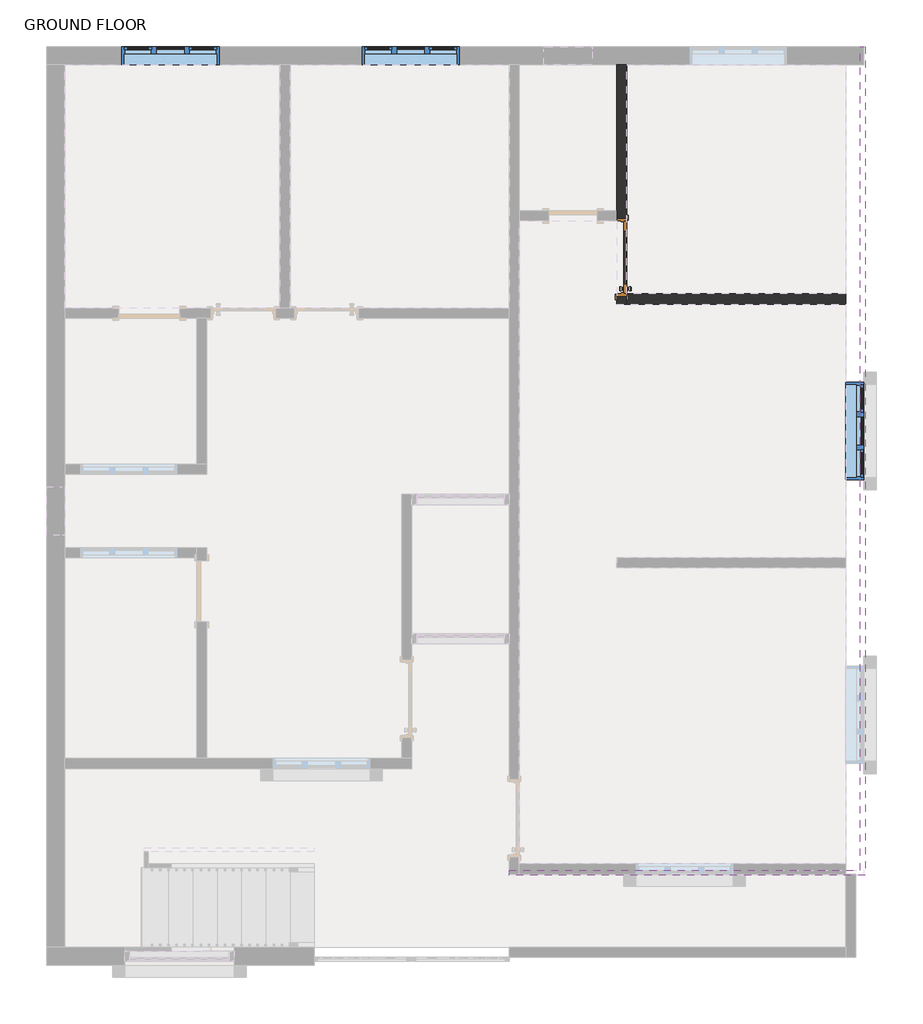
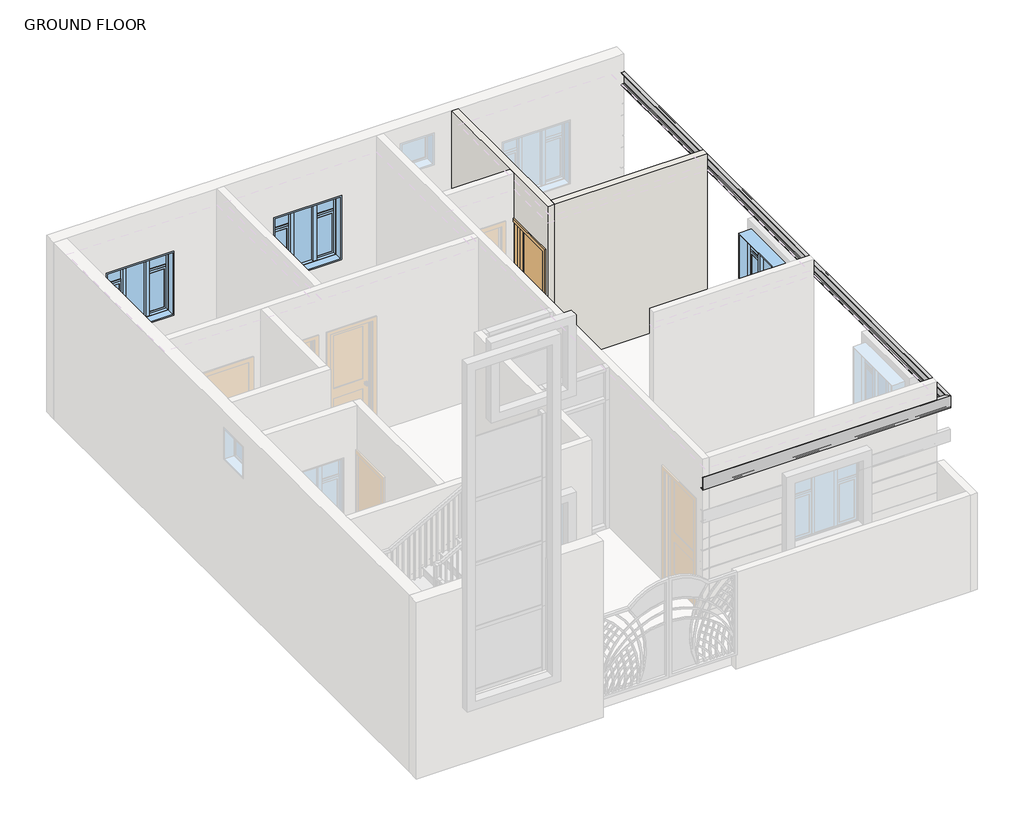
# One storey, part 4 of 7: 3 windows, 2 walls, 1 door, 1 proxy.
"""IFC4 building model written with IfcOpenShell, lengths in millimetres."""

from ifc_helpers import new_model, si_unit, frame, origin, place, context, project, spatial, polyline, circle_curve, ellipse_curve, faceted_brep, transform, mapped, element, save
from ifc_brep_helpers import plane_surface, cylinder_surface, revolved_surface, advanced_brep
from components import door_2e56f206, window_casement_triple_side_transom_window_4_x_4_fd24aed3

model = new_model("IFC4")

# Units and contexts
model_context = context("Model", 3, world=origin())
ifc_project = project(units=[si_unit("LENGTHUNIT", "METRE", prefix="MILLI")], contexts=[model_context])

# Site, building, storey
site = spatial("IfcSite", under=ifc_project)
building = spatial("IfcBuilding", under=site)
storey = spatial("IfcBuildingStorey", under=building, Name="GROUND FLOOR", Elevation=304.8)

# Proxy
placement = place(None, origin())
element("IfcBuildingElementProxy", 1, Name="Reveal", ObjectType="Reveal", at=placement, inside=storey, context=model_context, shape_type="AdvancedBrep", body=[
    advanced_brep(
    [(-9198.1023867, -1857.2343863, 3009.9), (-9198.1023867, -1793.9883863, 3009.9), (-9198.1023867, -1793.9883863, 3008.5203242), (-9198.1023867, -1798.3711955, 3003.3465897), (-9198.1023867, -1821.9918863, 2999.4098), (-9198.1023867, -1841.2297679, 2996.20348), (-9198.1023867, -1849.9953863, 2985.856011), (-9198.1023867, -1849.9953863, 2805.343989), (-9198.1023867, -1841.2297679, 2794.99652), (-9198.1023867, -1821.9918863, 2791.7902), (-9198.1023867, -1798.3711955, 2787.8534103), (-9198.1023867, -1793.9883863, 2782.6796758), (-9198.1023867, -1793.9883863, 2781.3), (-9198.1023867, -1857.2343863, 2781.3), (-4738.2179867, -1857.2343863, 3009.9), (-4738.2179867, -1857.2343863, 2781.3), (-4801.4639867, -1793.9883863, 2781.3), (-4801.4639867, -1793.9883863, 2782.6796758), (-4797.0811775, -1798.3711955, 2787.8534103), (-4773.4604867, -1821.9918863, 2791.7902), (-4754.2226051, -1841.2297679, 2794.99652), (-4745.4569867, -1849.9953863, 2805.343989), (-4745.4569867, -1849.9953863, 2985.856011), (-4754.2226051, -1841.2297679, 2996.20348), (-4773.4604867, -1821.9918863, 2999.4098), (-4797.0811775, -1798.3711955, 3003.3465897), (-4801.4639867, -1793.9883863, 3008.5203242), (-4801.4639867, -1793.9883863, 3009.9)],
    [
        (0, 1),
        (1, 2),
        (2, 3, circle_curve(frame((-9198.1023867, -1799.2334863, 3008.5203242), z_axis=(-1.0, 0.0, 0.0), x_axis=(0.0, 1.0, 0.0)), 5.2451)),
        (3, 4),
        (4, 5),
        (5, 6, circle_curve(frame((-9198.1023867, -1839.5051863, 2985.856011), z_axis=(1.0, 0.0, 0.0), x_axis=(0.0, 1.0, 0.0)), 10.4902)),
        (6, 7),
        (7, 8, circle_curve(frame((-9198.1023867, -1839.5051863, 2805.343989), z_axis=(1.0, 0.0, 0.0), x_axis=(0.0, 1.0, 0.0)), 10.4902)),
        (8, 9),
        (9, 10),
        (10, 11, circle_curve(frame((-9198.1023867, -1799.2334863, 2782.6796758), z_axis=(-1.0, 0.0, 0.0), x_axis=(0.0, 1.0, 0.0)), 5.2451)),
        (11, 12),
        (12, 13),
        (13, 0),
        (14, 15),
        (15, 16),
        (16, 17),
        (17, 18, ellipse_curve(frame((-4796.2188867, -1799.2334863, 2782.6796758), z_axis=(0.7071067811865498, 0.7071067811865454, 0.0), x_axis=(-0.7071067811865451, 0.7071067811865498, 0.0)), 7.4176916, 5.2451)),
        (18, 19),
        (19, 20),
        (20, 21, ellipse_curve(frame((-4755.9471867, -1839.5051863, 2805.343989), z_axis=(-0.7071067811865498, -0.7071067811865454, 0.0), x_axis=(0.7071067811865451, -0.7071067811865498, 0.0)), 14.8353831, 10.4902)),
        (21, 22),
        (22, 23, ellipse_curve(frame((-4755.9471867, -1839.5051863, 2985.856011), z_axis=(-0.7071067811865498, -0.7071067811865454, 0.0), x_axis=(0.7071067811865451, -0.7071067811865498, 0.0)), 14.8353831, 10.4902)),
        (23, 24),
        (24, 25),
        (25, 26, ellipse_curve(frame((-4796.2188867, -1799.2334863, 3008.5203242), z_axis=(0.7071067811865498, 0.7071067811865454, 0.0), x_axis=(-0.7071067811865451, 0.7071067811865498, 0.0)), 7.4176916, 5.2451)),
        (26, 27),
        (27, 14),
        (0, 14),
        (27, 1),
        (26, 2),
        (25, 3),
        (24, 4),
        (23, 5),
        (22, 6),
        (21, 7),
        (20, 8),
        (19, 9),
        (18, 10),
        (17, 11),
        (16, 12),
        (15, 13),
    ],
    [
        plane_surface(frame((-9198.1023867, 8292.2500137, 304.8), z_axis=(-1.0, 0.0, 0.0), x_axis=(0.0, -1.0, 0.0))),
        plane_surface(frame((-4753.1023867, -1842.3499863, 2590.8), z_axis=(0.7071067811865498, 0.7071067811865454, 0.0), x_axis=(-0.7071067811865454, 0.7071067811865498, 0.0))),
        plane_surface(frame((-9198.1023867, -1857.2343863, 3009.9), z_axis=(0.0, 0.0, 1.0), x_axis=(1.0, 0.0, 0.0))),
        plane_surface(frame((-9198.1023867, -1793.9883863, 3009.9), z_axis=(0.0, 1.0, 0.0), x_axis=(1.0, 0.0, 0.0))),
        cylinder_surface(frame((-9198.1023867, -1799.2334863, 3008.5203242), z_axis=(-1.0, 0.0, 0.0), x_axis=(0.0, 1.0, 0.0)), 5.2451),
        plane_surface(frame((-9198.1023867, -1798.3711955, 3003.3465897), z_axis=(0.0, 0.16439930721687082, -0.9863938705135049), x_axis=(1.0, 0.0, 0.0))),
        plane_surface(frame((-9198.1023867, -1821.9918863, 2999.4098), z_axis=(0.0, 0.16439930721687146, -0.9863938705135048), x_axis=(1.0, 0.0, 0.0))),
        revolved_surface(polyline([(-4745.4569867, -1829.0149863000001, 2985.856011), (-9198.1023867, -1829.0149863000001, 2985.856011)]), (-9198.1023867, -1839.5051863, 2985.856011), (1.0, 0.0, 0.0)),
        plane_surface(frame((-9198.1023867, -1849.9953863, 2985.856011), z_axis=(0.0, 1.0, 0.0), x_axis=(1.0, 0.0, 0.0))),
        revolved_surface(polyline([(-4745.4569867, -1829.0149863000001, 2805.343989), (-9198.1023867, -1829.0149863000001, 2805.343989)]), (-9198.1023867, -1839.5051863, 2805.343989), (1.0, 0.0, 0.0)),
        plane_surface(frame((-9198.1023867, -1841.2297679, 2794.99652), z_axis=(0.0, 0.1643993072168769, 0.9863938705135039), x_axis=(1.0, 0.0, 0.0))),
        plane_surface(frame((-9198.1023867, -1821.9918863, 2791.7902), z_axis=(0.0, 0.16439930721687793, 0.9863938705135037), x_axis=(1.0, 0.0, 0.0))),
        cylinder_surface(frame((-9198.1023867, -1799.2334863, 2782.6796758), z_axis=(-1.0, 0.0, 0.0), x_axis=(0.0, 1.0, 0.0)), 5.2451),
        plane_surface(frame((-9198.1023867, -1793.9883863, 2782.6796758), z_axis=(0.0, 1.0, 0.0), x_axis=(1.0, 0.0, 0.0))),
        plane_surface(frame((-9198.1023867, -1793.9883863, 2781.3), z_axis=(0.0, 0.0, -1.0), x_axis=(1.0, 0.0, 0.0))),
        plane_surface(frame((-9198.1023867, -1857.2343863, 2781.3), z_axis=(0.0, -1.0, 0.0), x_axis=(1.0, 0.0, 0.0))),
    ],
    [
        (0, [[1, 2, 3, 4, 5, 6, 7, 8, 9, 10, 11, 12, 13, 14]]),
        (1, [[15, 16, 17, 18, 19, 20, 21, 22, 23, 24, 25, 26, 27, 28]]),
        (2, [[-1, 29, -28, 30]]),
        (3, [[-2, -30, -27, 31]]),
        (4, [[-3, -31, -26, 32]]),
        (5, [[-4, -32, -25, 33]]),
        (6, [[-5, -33, -24, 34]]),
        (7, [[-6, -34, -23, 35]]),
        (8, [[-7, -35, -22, 36]]),
        (9, [[-8, -36, -21, 37]]),
        (10, [[-9, -37, -20, 38]]),
        (11, [[-10, -38, -19, 39]]),
        (12, [[-11, -39, -18, 40]]),
        (13, [[-12, -40, -17, 41]]),
        (14, [[-13, -41, -16, 42]]),
        (15, [[-14, -42, -15, -29]]),
    ],
),
    advanced_brep(
    [(-4738.2179867, 8520.8500137, 3009.9), (-4738.2179867, 8520.8500137, 2781.3), (-4801.4639867, 8520.8500137, 2781.3), (-4801.4639867, 8520.8500137, 2782.6796758), (-4797.0811775, 8520.8500137, 2787.8534103), (-4773.4604867, 8520.8500137, 2791.7902), (-4754.2226051, 8520.8500137, 2794.99652), (-4745.4569867, 8520.8500137, 2805.343989), (-4745.4569867, 8520.8500137, 2985.856011), (-4754.2226051, 8520.8500137, 2996.20348), (-4773.4604867, 8520.8500137, 2999.4098), (-4797.0811775, 8520.8500137, 3003.3465897), (-4801.4639867, 8520.8500137, 3008.5203242), (-4801.4639867, 8520.8500137, 3009.9), (-4738.2179867, -1857.2343863, 3009.9), (-4801.4639867, -1793.9883863, 3009.9), (-4801.4639867, -1793.9883863, 3008.5203242), (-4797.0811775, -1798.3711955, 3003.3465897), (-4773.4604867, -1821.9918863, 2999.4098), (-4754.2226051, -1841.2297679, 2996.20348), (-4745.4569867, -1849.9953863, 2985.856011), (-4745.4569867, -1849.9953863, 2805.343989), (-4754.2226051, -1841.2297679, 2794.99652), (-4773.4604867, -1821.9918863, 2791.7902), (-4797.0811775, -1798.3711955, 2787.8534103), (-4801.4639867, -1793.9883863, 2782.6796758), (-4801.4639867, -1793.9883863, 2781.3), (-4738.2179867, -1857.2343863, 2781.3)],
    [
        (0, 1),
        (1, 2),
        (2, 3),
        (3, 4, circle_curve(frame((-4796.2188867, 8520.8500137, 2782.6796758), z_axis=(0.0, 1.0, 0.0), x_axis=(-1.0, 0.0, 0.0)), 5.2451)),
        (4, 5),
        (5, 6),
        (6, 7, circle_curve(frame((-4755.9471867, 8520.8500137, 2805.343989), z_axis=(0.0, -1.0, 0.0), x_axis=(-1.0, 0.0, 0.0)), 10.4902)),
        (7, 8),
        (8, 9, circle_curve(frame((-4755.9471867, 8520.8500137, 2985.856011), z_axis=(0.0, -1.0, 0.0), x_axis=(-1.0, 0.0, 0.0)), 10.4902)),
        (9, 10),
        (10, 11),
        (11, 12, circle_curve(frame((-4796.2188867, 8520.8500137, 3008.5203242), z_axis=(0.0, 1.0, 0.0), x_axis=(-1.0, 0.0, 0.0)), 5.2451)),
        (12, 13),
        (13, 0),
        (14, 15),
        (15, 16),
        (16, 17, ellipse_curve(frame((-4796.2188867, -1799.2334863, 3008.5203242), z_axis=(-0.7071067811865498, -0.7071067811865454, 0.0), x_axis=(-0.7071067811865455, 0.7071067811865496, 0.0)), 7.4176916, 5.2451)),
        (17, 18),
        (18, 19),
        (19, 20, ellipse_curve(frame((-4755.9471867, -1839.5051863, 2985.856011), z_axis=(0.7071067811865498, 0.7071067811865454, 0.0), x_axis=(0.7071067811865455, -0.7071067811865496, 0.0)), 14.8353831, 10.4902)),
        (20, 21),
        (21, 22, ellipse_curve(frame((-4755.9471867, -1839.5051863, 2805.343989), z_axis=(0.7071067811865498, 0.7071067811865454, 0.0), x_axis=(0.7071067811865455, -0.7071067811865496, 0.0)), 14.8353831, 10.4902)),
        (22, 23),
        (23, 24),
        (24, 25, ellipse_curve(frame((-4796.2188867, -1799.2334863, 2782.6796758), z_axis=(-0.7071067811865498, -0.7071067811865454, 0.0), x_axis=(-0.7071067811865455, 0.7071067811865496, 0.0)), 7.4176916, 5.2451)),
        (25, 26),
        (26, 27),
        (27, 14),
        (0, 14),
        (27, 1),
        (26, 2),
        (25, 3),
        (24, 4),
        (23, 5),
        (22, 6),
        (21, 7),
        (20, 8),
        (19, 9),
        (18, 10),
        (17, 11),
        (16, 12),
        (15, 13),
    ],
    [
        plane_surface(frame((-14983.6015581, 8520.8500137, 0.0), z_axis=(0.0, 1.0, 0.0), x_axis=(-1.0, 0.0, 0.0))),
        plane_surface(frame((-4753.1023867, -1842.3499863, 3200.4), z_axis=(-0.7071067811865498, -0.7071067811865454, 0.0), x_axis=(-0.7071067811865454, 0.7071067811865498, 0.0))),
        plane_surface(frame((-4738.2179867, 8520.8500137, 3009.9), z_axis=(1.0, 0.0, 0.0), x_axis=(0.0, -1.0, 0.0))),
        plane_surface(frame((-4738.2179867, 8520.8500137, 2781.3), z_axis=(0.0, 0.0, -1.0), x_axis=(0.0, -1.0, 0.0))),
        plane_surface(frame((-4801.4639867, 8520.8500137, 2781.3), z_axis=(-1.0, 0.0, 0.0), x_axis=(0.0, -1.0, 0.0))),
        cylinder_surface(frame((-4796.2188867, 8520.8500137, 2782.6796758), z_axis=(0.0, 1.0, 0.0), x_axis=(-1.0, 0.0, 0.0)), 5.2451),
        plane_surface(frame((-4797.0811775, 8520.8500137, 2787.8534103), z_axis=(-0.16439930721687793, 0.0, 0.9863938705135037), x_axis=(0.0, -1.0, 0.0))),
        plane_surface(frame((-4773.4604867, 8520.8500137, 2791.7902), z_axis=(-0.1643993072168769, 0.0, 0.9863938705135039), x_axis=(0.0, -1.0, 0.0))),
        revolved_surface(polyline([(-4766.4373867, -1849.9953862999992, 2805.343989), (-4766.4373867, 8520.8500137, 2805.343989)]), (-4755.9471867, 8520.8500137, 2805.343989), (0.0, -1.0, 0.0)),
        plane_surface(frame((-4745.4569867, 8520.8500137, 2805.343989), z_axis=(-1.0, 0.0, 0.0), x_axis=(0.0, -1.0, 0.0))),
        revolved_surface(polyline([(-4766.4373867, -1849.9953862999992, 2985.856011), (-4766.4373867, 8520.8500137, 2985.856011)]), (-4755.9471867, 8520.8500137, 2985.856011), (0.0, -1.0, 0.0)),
        plane_surface(frame((-4754.2226051, 8520.8500137, 2996.20348), z_axis=(-0.16439930721687146, 0.0, -0.9863938705135048), x_axis=(0.0, -1.0, 0.0))),
        plane_surface(frame((-4773.4604867, 8520.8500137, 2999.4098), z_axis=(-0.16439930721687082, 0.0, -0.9863938705135049), x_axis=(0.0, -1.0, 0.0))),
        cylinder_surface(frame((-4796.2188867, 8520.8500137, 3008.5203242), z_axis=(0.0, 1.0, 0.0), x_axis=(-1.0, 0.0, 0.0)), 5.2451),
        plane_surface(frame((-4801.4639867, 8520.8500137, 3008.5203242), z_axis=(-1.0, 0.0, 0.0), x_axis=(0.0, -1.0, 0.0))),
        plane_surface(frame((-4801.4639867, 8520.8500137, 3009.9), z_axis=(0.0, 0.0, 1.0), x_axis=(0.0, -1.0, 0.0))),
    ],
    [
        (0, [[1, 2, 3, 4, 5, 6, 7, 8, 9, 10, 11, 12, 13, 14]]),
        (1, [[15, 16, 17, 18, 19, 20, 21, 22, 23, 24, 25, 26, 27, 28]]),
        (2, [[-1, 29, -28, 30]]),
        (3, [[-2, -30, -27, 31]]),
        (4, [[-3, -31, -26, 32]]),
        (5, [[-4, -32, -25, 33]]),
        (6, [[-5, -33, -24, 34]]),
        (7, [[-6, -34, -23, 35]]),
        (8, [[-7, -35, -22, 36]]),
        (9, [[-8, -36, -21, 37]]),
        (10, [[-9, -37, -20, 38]]),
        (11, [[-10, -38, -19, 39]]),
        (12, [[-11, -39, -18, 40]]),
        (13, [[-12, -40, -17, 41]]),
        (14, [[-13, -41, -16, 42]]),
        (15, [[-14, -42, -15, -29]]),
    ],
),
])

# Door
door_shape = door_2e56f206(model_context)
element("IfcDoor", 2, ObjectType="Door-Interior-Single-2_Panel-Wood : 36\" x 84\"", at=placement, inside=storey, context=model_context, shape_type="MappedRepresentation", body=[
    mapped(door_shape, transform((-7785.2273867, 5879.2500137, 304.8), x_axis=(0.0, 1.0, 0.0), y_axis=(-1.0, 0.0, 0.0), z_axis=(0.0, 0.0, 1.0))),
])

# Walls
element("IfcWall", 3, ObjectType="INNER WALL 5\"", at=placement, inside=storey, context=model_context, shape_type="Brep", body=[
    faceted_brep([(-7851.9023867, 5295.0500137, 3352.8), (-7851.9023867, 6336.4500137, 3352.8), (-7851.9023867, 6463.4500137, 3352.8), (-7851.9023867, 8292.2500137, 3352.8), (-7851.9023867, 8292.2500137, 304.8), (-7851.9023867, 6463.4500137, 304.8), (-7851.9023867, 6361.8500137, 304.8), (-7851.9023867, 6361.8500137, 2463.8), (-7851.9023867, 5396.6500137, 2463.8), (-7851.9023867, 5396.6500137, 304.8), (-7851.9023867, 5295.0500137, 304.8), (-7724.9023867, 8292.2500137, 3352.8), (-7724.9023867, 5422.0500137, 3352.8), (-7724.9023867, 5295.0500137, 3352.8), (-7724.9023867, 5295.0500137, 304.8), (-7724.9023867, 5396.6500137, 304.8), (-7724.9023867, 5396.6500137, 2463.8), (-7724.9023867, 6361.8500137, 2463.8), (-7724.9023867, 6361.8500137, 304.8), (-7724.9023867, 8292.2500137, 304.8)], [[[0, 1, 2, 3, 4, 5, 6, 7, 8, 9, 10]], [[11, 12, 13, 14, 15, 16, 17, 18, 19]], [[4, 19, 18, 6, 5]], [[14, 10, 9, 15]], [[3, 2, 1, 0, 13, 12, 11]], [[4, 3, 11, 19]], [[0, 10, 14, 13]], [[17, 7, 6, 18]], [[7, 17, 16, 8]], [[8, 16, 15, 9]]]),
])
element("IfcWall", 4, ObjectType="INNER WALL 5\"", at=placement, inside=storey, context=model_context, shape_type="Brep", body=[
    faceted_brep([(-4981.7023867, 5422.0500137, 304.8), (-7724.9023867, 5422.0500137, 304.8), (-7724.9023867, 5422.0500137, 3352.8), (-4981.7023867, 5422.0500137, 3352.8), (-4981.7023867, 5295.0500137, 304.8), (-4981.7023867, 5295.0500137, 3352.8), (-7724.9023867, 5295.0500137, 3352.8), (-7724.9023867, 5295.0500137, 304.8), (-7724.9023867, 5396.6500137, 304.8)], [[[0, 1, 2, 3]], [[4, 5, 6, 7]], [[1, 0, 4, 7, 8]], [[3, 2, 6, 5]], [[2, 1, 8, 7, 6]], [[0, 3, 5, 4]]]),
])

# Windows
window_casement_triple_side_transom_window_4_x_4_shape = window_casement_triple_side_transom_window_4_x_4_fd24aed3(model_context)
element("IfcWindow", 5, ObjectType="Window-Casement-Triple-Side-Transom : window 4' x 4'", at=placement, inside=storey, context=model_context, shape_type="MappedRepresentation", body=[
    mapped(window_casement_triple_side_transom_window_4_x_4_shape, transform((-13439.9023867, 8406.5500137, 304.8), x_axis=(1.0, 0.0, 0.0), y_axis=(0.0, 1.0, 0.0), z_axis=(0.0, 0.0, 1.0))),
])
element("IfcWindow", 6, ObjectType="Window-Casement-Triple-Side-Transom : window 4' x 4'", at=placement, inside=storey, context=model_context, shape_type="MappedRepresentation", body=[
    mapped(window_casement_triple_side_transom_window_4_x_4_shape, transform((-10430.0023867, 8406.5500137, 304.8), x_axis=(1.0, 0.0, 0.0), y_axis=(0.0, 1.0, 0.0), z_axis=(0.0, 0.0, 1.0))),
])
element("IfcWindow", 7, ObjectType="Window-Casement-Triple-Side-Transom : window 4' x 4'", at=placement, inside=storey, context=model_context, shape_type="MappedRepresentation", body=[
    mapped(window_casement_triple_side_transom_window_4_x_4_shape, transform((-4867.4023867, 3707.5500137, 304.8), x_axis=(0.0, -1.0, 0.0), y_axis=(1.0, 0.0, 0.0), z_axis=(0.0, 0.0, 1.0))),
])

save(model, "model.ifc")

# Revit data of these elements
# Type "Door-Interior-Single-2_Panel-Wood : 36\" x 84\""
#   Type Mark = "8"
#   Assembly Code = "C1020300"
#   Analytic Construction = "Wooden"
#   Top Rail = 0' - 4 11/16"
#   Thickness = 0' - 1 3/8"
#   Thermal Resistance (R) = 2.5876 (h·ft²·°F)/BTU
#   Swing Angle [instance default] = 90.00°
#   Stiles = 0' - 4 3/4"
#   Rough Width = 3' - 2"
#   Rough Height = 7' - 1"
#   Lock Rail = 0' - 7 1/2"
#   Height = 7' - 0"
#   Width = 3' - 0"
#   Heat Transfer Coefficient (U) = 0.3865 BTU/(h·ft²·°F)
#   Bottom Rail = 0' - 9 1/8"
#   Trim Material = Cherry
#   Panel Material = Cherry
#   Frame Material = Cherry
#   Door Handle Material = Aluminum
#   Visual Light Transmittance = 0
#   Solar Heat Gain Coefficient = 0
#   Wall Closure = (empty or 0)
#   Function = (empty or 0)
# Type "INNER WALL 5\""
#   Assembly Code = "B2010"
#   Layers, outside or top first: 0' - 5" "OUTER WALL" (function 1)
# Type "Window-Casement-Triple-Side-Transom : window 4' x 4'"
#   Type Mark = "22"
#   Fire Rating = "0.5h"
#   Assembly Code = "B2020100"
#   Analytic Construction = "Double glazing - domestic"
#   Window Width = 1' - 4"
#   Window Inset [instance default] = 0' - 0 5/8"
#   Wall Thickness [instance default] = 0' - 6"
#   Visual Light Transmittance = 0.81
#   Transom Height Ratio = 0.3
#   Thermal Resistance (R) = 1.8146 (h·ft²·°F)/BTU
#   Solar Heat Gain Coefficient = 0.76
#   Rough Width = 4' - 0 1/2"
#   Rough Height = 4' - 0 1/2"
#   Open Window Height = 2' - 9.6"
#   Heat Transfer Coefficient (U) = 0.5511 BTU/(h·ft²·°F)
#   Height = 4' - 0"
#   Transom Height = 1' - 2.4"
#   Frame Gap 3 [instance default] = 0' - 1 83/128"
#   Frame Gap 2 [instance default] = 0' - 0 5/8"
#   Frame Gap 1 = 0' - 1 51/128"
#   Default Sill Height = 3' - 0"
#   Width = 4' - 0"
#   Frame Material = Metal - Aluminum
#   Glass Panel Material = Glass
#   Wall Closure = (empty or 0)
# Element 2 (IfcDoor, "Door-Interior-Single-2_Panel-Wood : 36\" x 84\"")
#   Swing Angle = 90.00°
#   Phase Created = New Construction
#   Materials on its faces: "Cherry", "Aluminum"
# Elements 3, 4 (IfcWall, "INNER WALL 5\"")
#   Top Offset = 0' - 0"
#   Base Offset = 0' - 0"
#   wall height = 10' - 0"
#   Phase Created = New Construction
#   Base Constraint = GROUND FLOOR
#   Top Constraint = FIRST FLOOR
#   Materials on its faces: "OUTER WALL"
# Element 5 (IfcWindow, "Window-Casement-Triple-Side-Transom : window 4' x 4'")
#   Mark = "5"
#   Window Inset = 0' - 0 5/8"
#   Frame Gap 3 = 0' - 1 83/128"
#   Frame Gap 2 = 0' - 0 5/8"
#   Phase Created = New Construction
#   Materials on its faces: "Metal - Aluminum", "Glass"
# Element 6 (IfcWindow, "Window-Casement-Triple-Side-Transom : window 4' x 4'")
#   Mark = "6"
#   Window Inset = 0' - 0 5/8"
#   Frame Gap 3 = 0' - 1 83/128"
#   Frame Gap 2 = 0' - 0 5/8"
#   Phase Created = New Construction
#   Materials on its faces: "Metal - Aluminum", "Glass"
# Element 7 (IfcWindow, "Window-Casement-Triple-Side-Transom : window 4' x 4'")
#   Mark = "10"
#   Window Inset = 0' - 0 5/8"
#   Frame Gap 3 = 0' - 1 83/128"
#   Frame Gap 2 = 0' - 0 5/8"
#   Phase Created = New Construction
#   Materials on its faces: "Metal - Aluminum", "Glass"
# Materials
#   "Cherry": class "Wood", colour RGB 226 177 128, transparency 0, Description = "Prunus Serotina", Cost = 0
#   "Aluminum": class "Metal", colour RGB 247 247 247, transparency 0, Description = "Aluminum 6061", Cost = 0
#   "OUTER WALL": class "Generic", colour RGB 245 245 240, transparency 0, Cost = 0
#   "Metal - Aluminum": class "Metal", colour RGB 247 247 247, transparency 0
#   "Glass": class "Glass", colour RGB 0 128 192, transparency 0.75, Description = "Soda Lime Glass", Cost = 0
